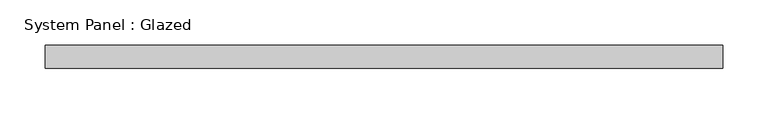
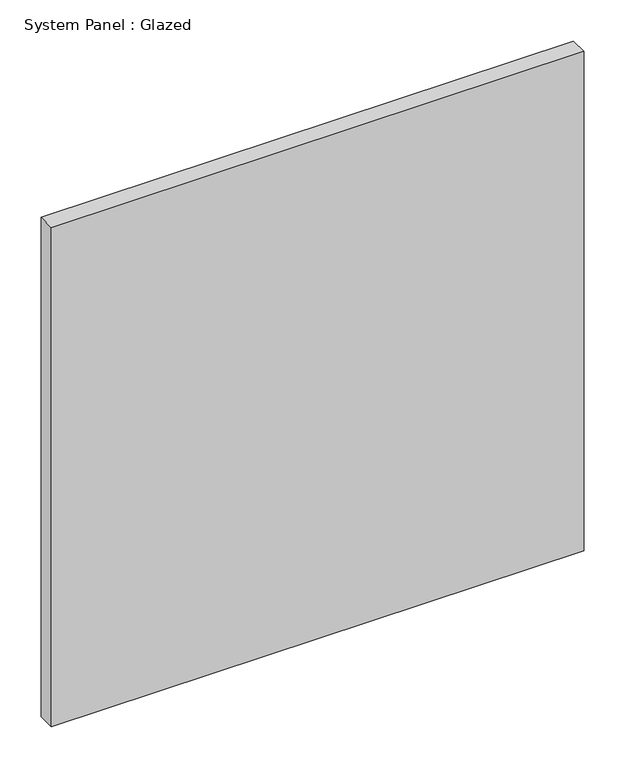
"""IFC4 building model written with IfcOpenShell, lengths in millimetres: plate geometry, System Panel : Glazed."""

from ifc_helpers import new_model, si_unit, origin, origin_with_axes, place, context, project, spatial, polyline, outline, extrude, source, transform, mapped, element, save


def system_panel_glazed_a2941881(model_context):
    return source(origin(), model_context, "Body", "SweptSolid", [
        extrude(outline(polyline([(374.65, 19.05), (-374.65, 19.05), (-374.65, 44.45), (374.65, 44.45), (374.65, 19.05)])), origin_with_axes(), (0.0, 0.0, 1.0), 742.6074877),
    ])


if __name__ == "__main__":
    model = new_model("IFC4")
    model_context = context("Model", 3, world=origin())
    ifc_project = project(units=[si_unit("LENGTHUNIT", "METRE", prefix="MILLI")], contexts=[model_context])
    site = spatial("IfcSite", under=ifc_project)
    building = spatial("IfcBuilding", under=site)
    placement = place(None, origin())
    system_panel_glazed_shape = system_panel_glazed_a2941881(model_context)
    element("IfcPlate", 1, ObjectType="System Panel : Glazed", at=placement, inside=building, context=model_context, shape_type="MappedRepresentation", body=[
        mapped(system_panel_glazed_shape, transform((0.0, 0.0, 0.0), x_axis=(1.0, 0.0, 0.0), y_axis=(0.0, 1.0, 0.0), z_axis=(0.0, 0.0, 1.0))),
    ])
    save(model, "model.ifc")

# Revit data of these elements
# Type "System Panel : Glazed"
#   Construction Type Id = "GSP4R"
#   Analytic Construction = "1/8 in Pilkington single glazing"
#   Visual Light Transmittance = 0.9
#   Solar Heat Gain Coefficient = 0.86
#   Heat Transfer Coefficient (U) = 1.18115 BTU/(h·ft²·°F)
#   Define Thermal Properties by = 1
# Element 1 (IfcPlate, "System Panel : Glazed")
#   Materials on its faces: "Glass"
# Materials
#   "Glass": class "Glass", colour RGB 0 128 192, transparency 0.75, Description = "Soda Lime Glass", Cost = 0
